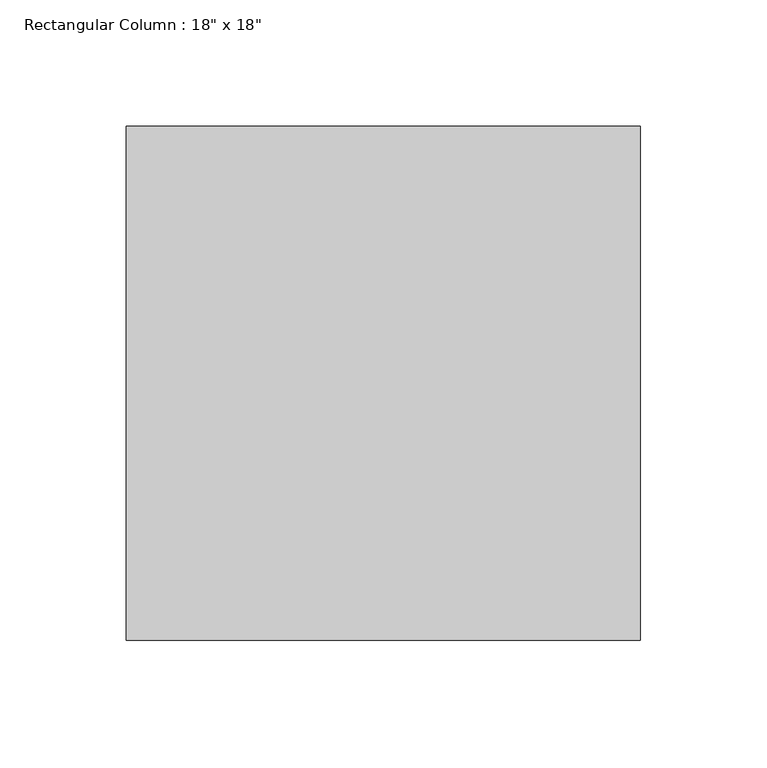
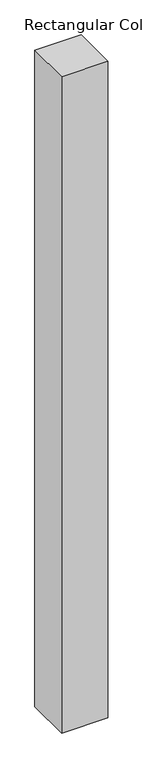
"""IFC4 building model written with IfcOpenShell, lengths in millimetres: column geometry."""

from ifc_helpers import new_model, si_unit, origin, origin_with_axes, place, context, project, spatial, polyline, outline, extrude, source, transform, mapped, element, save


def column_81985572(model_context):
    return source(origin(), model_context, "Body", "SweptSolid", [
        extrude(outline(polyline([(101.6, 101.6), (101.6, -101.6), (-101.6, -101.6), (-101.6, 101.6), (101.6, 101.6)])), origin_with_axes(), (0.0, 0.0, 1.0), 3048.0),
    ])


if __name__ == "__main__":
    model = new_model("IFC4")
    model_context = context("Model", 3, world=origin())
    ifc_project = project(units=[si_unit("LENGTHUNIT", "METRE", prefix="MILLI")], contexts=[model_context])
    site = spatial("IfcSite", under=ifc_project)
    building = spatial("IfcBuilding", under=site)
    placement = place(None, origin())
    column_shape = column_81985572(model_context)
    element("IfcColumn", 1, ObjectType="Rectangular Column : 18\" x 18\"", at=placement, inside=building, context=model_context, shape_type="MappedRepresentation", body=[
        mapped(column_shape, transform((0.0, 0.0, 0.0), x_axis=(1.0, 0.0, 0.0), y_axis=(0.0, 1.0, 0.0), z_axis=(0.0, 0.0, 1.0))),
    ])
    save(model, "model.ifc")

# Revit data of these elements
# Type "Rectangular Column : 18\" x 18\""
#   Assembly Code = "B1010200"
#   Depth = 0' - 8"
#   Offset Base = 0' - 0"
#   Offset Top = 0' - 0"
#   Width = 0' - 8"
#   Material = Stainless Steel
# Element 1 (IfcColumn, "Rectangular Column : 18\" x 18\"")
#   Materials on its faces: "Stainless Steel"
# Materials
#   "Stainless Steel": class "Metal", colour RGB 0 0 0, transparency 0, Description = "Stainless Steel 18/8", Cost = 0
